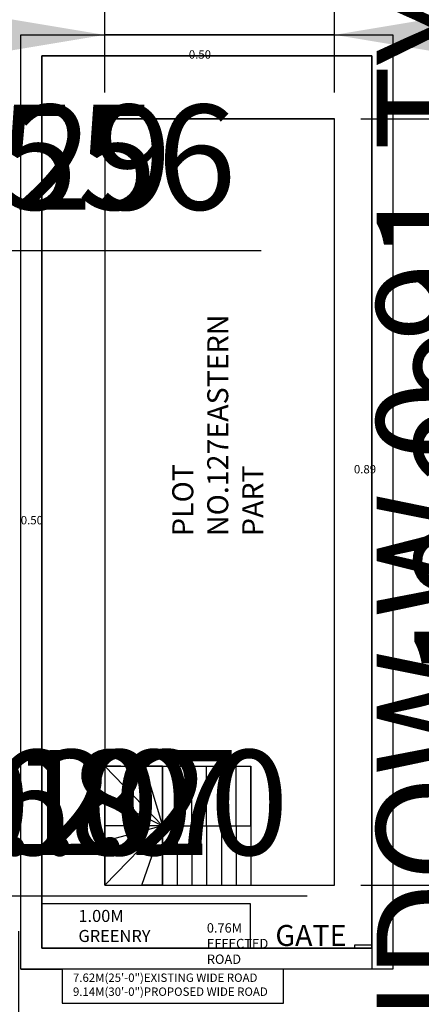
# Model space of a CAD drawing. Units: metres. Extents: x 782 to 1487, y 1262 to 7446.
# Tile 22 of 25: x 816.33 to 825.91, y 1313.5 to 1336.99. Entities that reach past the tile are written whole.
import ezdxf

# ---------------------------------------------------------------- set-up
doc = ezdxf.new("R2010")
doc.units = ezdxf.units.M
for name, color, linetype, lineweight in [('A-ANNO-DIMS', 2, 'Continuous', 18), ('A-ANNO-TEXT', 3, 'Continuous', 18), ('C-PROP', 6, 'Continuous', 25)]:
    doc.layers.add(name, color=color, linetype=linetype, lineweight=lineweight)
doc.styles.get("Standard").update_dxf_attribs({"font": 'arial.ttf'})
doc.dimstyles.new('ISO-25', dxfattribs={"dimtxt": 2.5, "dimasz": 2.5, "dimexe": 1.25, "dimexo": 0.625, "dimtad": 1, "dimtxsty": 'Standard', "dimcen": 2.5, "dimadec": 0, "dimazin": 0, "dimtfac": 1, "dimtmove": 0, "dimatfit": 3, "dimfxl": 1, "dimarcsym": 0})

# ---------------------------------------------------------------- blocks, each defined once
blk = doc.blocks.new('*D11')
at = {"layer": 'A-ANNO-DIMS', "color": 0, "lineweight": -2, "transparency": 16777216}
for p, q in [((824.462, 1334.623), (830.687, 1334.623)), ((829.437, 1332.123), (829.437, 1318.837)), ((824.462, 1316.337), (830.687, 1316.337))]:
    blk.add_line(p, q, dxfattribs=at)
at = {"layer": 'A-ANNO-DIMS', "color": 0, "transparency": 16777216}
for points in [[(829.02, 1332.123), (829.854, 1332.123), (829.437, 1334.623)], [(829.02, 1318.837), (829.854, 1318.837), (829.437, 1316.337)]]:
    blk.add_solid(points, dxfattribs=at)
at = {"layer": 'Defpoints', "color": 0, "transparency": 16777216}
for p in [(823.837, 1334.623), (823.837, 1316.337), (829.437, 1316.337)]:
    blk.add_point(p, dxfattribs=at)
at = {"layer": 'A-ANNO-DIMS', "color": 0, "transparency": 16777216, "insert": (827.31, 1325.48), "char_height": 2.5, "attachment_point": 5, "rotation": 90}
blk.add_mtext('18,29', dxfattribs=at)
blk = doc.blocks.new('*D12')
at = {"layer": 'A-ANNO-DIMS', "color": 0, "lineweight": -2, "transparency": 16777216}
for p, q in [((818.357, 1335.252), (818.357, 1337.877)), ((823.837, 1335.252), (823.837, 1337.877)), ((815.857, 1336.627), (805.608, 1336.627)), ((823.837, 1336.627), (818.357, 1336.627)), ((826.337, 1336.627), (828.837, 1336.627))]:
    blk.add_line(p, q, dxfattribs=at)
at = {"layer": 'A-ANNO-DIMS', "color": 0, "transparency": 16777216}
for points in [[(815.857, 1337.044), (815.857, 1336.21), (818.357, 1336.627)], [(826.337, 1337.044), (826.337, 1336.21), (823.837, 1336.627)]]:
    blk.add_solid(points, dxfattribs=at)
at = {"layer": 'Defpoints', "color": 0, "transparency": 16777216}
for p in [(818.357, 1336.627), (818.357, 1334.627), (823.837, 1334.627)]:
    blk.add_point(p, dxfattribs=at)
at = {"layer": 'A-ANNO-DIMS', "color": 0, "transparency": 16777216, "insert": (809.482, 1338.754), "char_height": 2.5, "width": 6.51678, "attachment_point": 5}
blk.add_mtext('5,48', dxfattribs=at)
blk = doc.blocks.new('*D20')
at = {"layer": 'A-ANNO-DIMS', "color": 0, "lineweight": -2, "transparency": 16777216}
for p, q in [((831.056, 1302.088), (831.056, 1337.678)), ((831.056, 1298.698), (831.056, 1299.588)), ((831.548, 1299.588), (832.306, 1299.588)), ((831.548, 1298.698), (832.306, 1298.698)), ((831.056, 1296.198), (831.056, 1293.698))]:
    blk.add_line(p, q, dxfattribs=at)
at = {"layer": 'A-ANNO-DIMS', "color": 0, "transparency": 16777216}
for points in [[(830.64, 1302.088), (831.473, 1302.088), (831.056, 1299.588)], [(830.64, 1296.198), (831.473, 1296.198), (831.056, 1298.698)]]:
    blk.add_solid(points, dxfattribs=at)
at = {"layer": 'Defpoints', "color": 0, "transparency": 16777216}
for p in [(830.923, 1299.588), (831.056, 1299.588), (830.923, 1298.698)]:
    blk.add_point(p, dxfattribs=at)
at = {"layer": 'A-ANNO-DIMS', "color": 0, "transparency": 16777216, "insert": (829.138, 1321.133), "char_height": 2.5, "attachment_point": 5, "rotation": 90}
blk.add_mtext('DOOR D1 0.89 TYP.', dxfattribs=at)
blk = doc.blocks.new('*D23')
at = {"layer": 'A-ANNO-DIMS', "color": 0, "lineweight": -2, "transparency": 16777216}
for p, q in [((816.313, 1296.414), (816.313, 1315.246)), ((816.313, 1293.067), (816.313, 1293.914)), ((816.804, 1293.914), (817.563, 1293.914)), ((816.804, 1293.067), (817.563, 1293.067)), ((816.313, 1290.567), (816.313, 1288.067))]:
    blk.add_line(p, q, dxfattribs=at)
at = {"layer": 'A-ANNO-DIMS', "color": 0, "transparency": 16777216}
for points in [[(815.896, 1296.414), (816.729, 1296.414), (816.313, 1293.914)], [(815.896, 1290.567), (816.729, 1290.567), (816.313, 1293.067)]]:
    blk.add_solid(points, dxfattribs=at)
at = {"layer": 'Defpoints', "color": 0, "transparency": 16777216}
for p in [(816.179, 1293.914), (816.313, 1293.914), (816.179, 1293.067)]:
    blk.add_point(p, dxfattribs=at)
at = {"layer": 'A-ANNO-DIMS', "color": 0, "transparency": 16777216, "insert": (814.411, 1307.08), "char_height": 2.5, "attachment_point": 5, "rotation": 90}
blk.add_mtext('0.85 TYP.', dxfattribs=at)
blk = doc.blocks.new('*D25')
at = {"layer": 'A-ANNO-DIMS', "color": 0, "lineweight": -2, "transparency": 16777216}
for p, q in [((814.687, 1297.897), (814.687, 1316.729)), ((814.687, 1294.551), (814.687, 1295.397)), ((815.184, 1295.397), (815.937, 1295.397)), ((815.184, 1294.551), (815.937, 1294.551)), ((814.687, 1292.051), (814.687, 1289.551))]:
    blk.add_line(p, q, dxfattribs=at)
at = {"layer": 'A-ANNO-DIMS', "color": 0, "transparency": 16777216}
for points in [[(814.27, 1297.897), (815.103, 1297.897), (814.687, 1295.397)], [(814.27, 1292.051), (815.103, 1292.051), (814.687, 1294.551)]]:
    blk.add_solid(points, dxfattribs=at)
at = {"layer": 'Defpoints', "color": 0, "transparency": 16777216}
for p in [(814.559, 1295.397), (814.687, 1295.397), (814.559, 1294.551)]:
    blk.add_point(p, dxfattribs=at)
at = {"layer": 'A-ANNO-DIMS', "color": 0, "transparency": 16777216, "insert": (812.785, 1308.563), "char_height": 2.5, "attachment_point": 5, "rotation": 90}
blk.add_mtext('0.85 TYP.', dxfattribs=at)
blk = doc.blocks.new('*D26')
at = {"layer": 'A-ANNO-DIMS', "color": 0, "lineweight": -2, "transparency": 16777216}
for p, q in [((828.33, 1303.223), (828.33, 1342.718)), ((828.33, 1299.809), (828.33, 1300.723)), ((828.818, 1300.723), (829.58, 1300.723)), ((828.818, 1299.809), (829.58, 1299.809)), ((828.33, 1297.309), (828.33, 1294.809))]:
    blk.add_line(p, q, dxfattribs=at)
at = {"layer": 'A-ANNO-DIMS', "color": 0, "transparency": 16777216}
for points in [[(827.913, 1303.223), (828.747, 1303.223), (828.33, 1300.723)], [(827.913, 1297.309), (828.747, 1297.309), (828.33, 1299.809)]]:
    blk.add_solid(points, dxfattribs=at)
at = {"layer": 'Defpoints', "color": 0, "transparency": 16777216}
for p in [(828.193, 1300.723), (828.33, 1300.723), (828.193, 1299.809)]:
    blk.add_point(p, dxfattribs=at)
at = {"layer": 'A-ANNO-DIMS', "color": 0, "transparency": 16777216, "insert": (826.412, 1324.22), "char_height": 2.5, "attachment_point": 5, "rotation": 90}
blk.add_mtext('WINDOW W 0.91 TYP.', dxfattribs=at)
blk = doc.blocks.new('*D28')
at = {"layer": 'A-ANNO-DIMS', "color": 0, "lineweight": -2, "transparency": 16777216}
for p, q in [((832.55, 1308.281), (832.55, 1349.718)), ((832.55, 1304.867), (832.55, 1305.781)), ((833.038, 1305.781), (833.8, 1305.781)), ((833.038, 1304.867), (833.8, 1304.867)), ((832.55, 1302.367), (832.55, 1299.867))]:
    blk.add_line(p, q, dxfattribs=at)
at = {"layer": 'A-ANNO-DIMS', "color": 0, "transparency": 16777216}
for points in [[(832.134, 1308.281), (832.967, 1308.281), (832.55, 1305.781)], [(832.134, 1302.367), (832.967, 1302.367), (832.55, 1304.867)]]:
    blk.add_solid(points, dxfattribs=at)
at = {"layer": 'Defpoints', "color": 0, "transparency": 16777216}
for p in [(832.413, 1305.781), (832.55, 1305.781), (832.413, 1304.867)]:
    blk.add_point(p, dxfattribs=at)
at = {"layer": 'A-ANNO-DIMS', "color": 0, "transparency": 16777216, "insert": (830.632, 1330.25), "char_height": 2.5, "attachment_point": 5, "rotation": 90}
blk.add_mtext('WINDOW W1 0.91 TYP.', dxfattribs=at)
blk = doc.blocks.new('*D137')
at = {"layer": 'A-ANNO-DIMS', "color": 0, "lineweight": -2, "transparency": 16777216}
for p, q in [((803.332, 1330.988), (803.332, 1332.733)), ((809.888, 1330.988), (809.888, 1332.733)), ((805.832, 1331.483), (807.388, 1331.483)), ((809.888, 1331.483), (822.086, 1331.483))]:
    blk.add_line(p, q, dxfattribs=at)
at = {"layer": 'A-ANNO-DIMS', "color": 0, "transparency": 16777216}
for points in [[(805.832, 1331.899), (805.832, 1331.066), (803.332, 1331.483)], [(807.388, 1331.899), (807.388, 1331.066), (809.888, 1331.483)]]:
    blk.add_solid(points, dxfattribs=at)
at = {"layer": 'Defpoints', "color": 0, "transparency": 16777216}
for p in [(809.888, 1331.483), (803.332, 1330.363), (809.888, 1330.363)]:
    blk.add_point(p, dxfattribs=at)
at = {"layer": 'A-ANNO-DIMS', "color": 0, "transparency": 16777216, "insert": (817.237, 1333.384), "char_height": 2.5, "attachment_point": 5}
blk.add_mtext('6.556', dxfattribs=at)
blk = doc.blocks.new('*D139')
at = {"layer": 'A-ANNO-DIMS', "color": 0, "lineweight": -2, "transparency": 16777216}
for p, q in [((807.481, 1330.074), (807.481, 1332.733)), ((807.769, 1330.074), (807.769, 1332.733)), ((804.981, 1331.483), (802.481, 1331.483)), ((807.481, 1331.483), (807.769, 1331.483)), ((810.269, 1331.483), (820.518, 1331.483))]:
    blk.add_line(p, q, dxfattribs=at)
at = {"layer": 'A-ANNO-DIMS', "color": 0, "transparency": 16777216}
for points in [[(804.981, 1331.899), (804.981, 1331.066), (807.481, 1331.483)], [(810.269, 1331.899), (810.269, 1331.066), (807.769, 1331.483)]]:
    blk.add_solid(points, dxfattribs=at)
at = {"layer": 'Defpoints', "color": 0, "transparency": 16777216}
for p in [(807.769, 1331.483), (807.481, 1329.449), (807.769, 1329.449)]:
    blk.add_point(p, dxfattribs=at)
at = {"layer": 'A-ANNO-DIMS', "color": 0, "transparency": 16777216, "insert": (816.644, 1333.384), "char_height": 2.5, "attachment_point": 5}
blk.add_mtext('0.29', dxfattribs=at)
blk = doc.blocks.new('*D140')
at = {"layer": 'A-ANNO-DIMS', "color": 0, "lineweight": -2, "transparency": 16777216}
for p, q in [((803.316, 1317.905), (803.316, 1314.838)), ((804.52, 1317.905), (804.52, 1314.838)), ((800.816, 1316.088), (798.316, 1316.088)), ((803.316, 1316.088), (804.52, 1316.088)), ((807.02, 1316.088), (817.02, 1316.088))]:
    blk.add_line(p, q, dxfattribs=at)
at = {"layer": 'A-ANNO-DIMS', "color": 0, "transparency": 16777216}
for points in [[(800.816, 1316.505), (800.816, 1315.671), (803.316, 1316.088)], [(807.02, 1316.505), (807.02, 1315.671), (804.52, 1316.088)]]:
    blk.add_solid(points, dxfattribs=at)
at = {"layer": 'Defpoints', "color": 0, "transparency": 16777216}
for p in [(803.316, 1318.53), (804.52, 1318.53), (804.52, 1316.088)]:
    blk.add_point(p, dxfattribs=at)
at = {"layer": 'A-ANNO-DIMS', "color": 0, "transparency": 16777216, "insert": (813.27, 1317.989), "char_height": 2.5, "attachment_point": 5}
blk.add_mtext('1.20', dxfattribs=at)
blk = doc.blocks.new('*D141')
at = {"layer": 'A-ANNO-DIMS', "color": 0, "lineweight": -2, "transparency": 16777216}
for p, q in [((804.52, 1317.905), (804.52, 1314.838)), ((807.205, 1317.905), (807.205, 1314.838)), ((802.02, 1316.088), (799.52, 1316.088)), ((804.52, 1316.088), (807.205, 1316.088)), ((809.705, 1316.088), (819.997, 1316.088))]:
    blk.add_line(p, q, dxfattribs=at)
at = {"layer": 'A-ANNO-DIMS', "color": 0, "transparency": 16777216}
for points in [[(802.02, 1316.505), (802.02, 1315.671), (804.52, 1316.088)], [(809.705, 1316.505), (809.705, 1315.671), (807.205, 1316.088)]]:
    blk.add_solid(points, dxfattribs=at)
at = {"layer": 'Defpoints', "color": 0, "transparency": 16777216}
for p in [(804.52, 1318.53), (807.205, 1318.53), (807.205, 1316.088)]:
    blk.add_point(p, dxfattribs=at)
at = {"layer": 'A-ANNO-DIMS', "color": 0, "transparency": 16777216, "insert": (816.101, 1317.989), "char_height": 2.5, "attachment_point": 5}
blk.add_mtext('2.68', dxfattribs=at)
blk = doc.blocks.new('*D142')
at = {"layer": 'A-ANNO-DIMS', "color": 0, "lineweight": -2, "transparency": 16777216}
for p, q in [((807.205, 1317.905), (807.205, 1314.838)), ((808.409, 1317.905), (808.409, 1314.838)), ((804.705, 1316.088), (802.205, 1316.088)), ((807.205, 1316.088), (808.409, 1316.088)), ((810.909, 1316.088), (820.909, 1316.088))]:
    blk.add_line(p, q, dxfattribs=at)
at = {"layer": 'A-ANNO-DIMS', "color": 0, "transparency": 16777216}
for points in [[(804.705, 1316.505), (804.705, 1315.671), (807.205, 1316.088)], [(810.909, 1316.505), (810.909, 1315.671), (808.409, 1316.088)]]:
    blk.add_solid(points, dxfattribs=at)
at = {"layer": 'Defpoints', "color": 0, "transparency": 16777216}
for p in [(807.205, 1318.53), (808.409, 1318.53), (808.409, 1316.088)]:
    blk.add_point(p, dxfattribs=at)
at = {"layer": 'A-ANNO-DIMS', "color": 0, "transparency": 16777216, "insert": (817.159, 1317.989), "char_height": 2.5, "attachment_point": 5}
blk.add_mtext('1.20', dxfattribs=at)
blk = doc.blocks.new('*D143')
at = {"layer": 'A-ANNO-DIMS', "color": 0, "lineweight": -2, "transparency": 16777216}
for p, q in [((808.409, 1317.905), (808.409, 1314.838)), ((809.479, 1317.905), (809.479, 1314.838)), ((805.909, 1316.088), (803.409, 1316.088)), ((808.409, 1316.088), (809.479, 1316.088)), ((811.979, 1316.088), (821.987, 1316.088))]:
    blk.add_line(p, q, dxfattribs=at)
at = {"layer": 'A-ANNO-DIMS', "color": 0, "transparency": 16777216}
for points in [[(805.909, 1316.505), (805.909, 1315.671), (808.409, 1316.088)], [(811.979, 1316.505), (811.979, 1315.671), (809.479, 1316.088)]]:
    blk.add_solid(points, dxfattribs=at)
at = {"layer": 'Defpoints', "color": 0, "transparency": 16777216}
for p in [(808.409, 1318.53), (809.479, 1318.53), (809.479, 1316.088)]:
    blk.add_point(p, dxfattribs=at)
at = {"layer": 'A-ANNO-DIMS', "color": 0, "transparency": 16777216, "insert": (818.233, 1317.989), "char_height": 2.5, "attachment_point": 5}
blk.add_mtext('1.07', dxfattribs=at)
blk = doc.blocks.new('*D144')
at = {"layer": 'A-ANNO-DIMS', "color": 0, "lineweight": -2, "transparency": 16777216}
for p, q in [((809.479, 1317.905), (809.479, 1314.838)), ((810.683, 1317.905), (810.683, 1314.838)), ((806.979, 1316.088), (804.479, 1316.088)), ((809.479, 1316.088), (810.683, 1316.088)), ((813.183, 1316.088), (823.183, 1316.088))]:
    blk.add_line(p, q, dxfattribs=at)
at = {"layer": 'A-ANNO-DIMS', "color": 0, "transparency": 16777216}
for points in [[(806.979, 1316.505), (806.979, 1315.671), (809.479, 1316.088)], [(813.183, 1316.505), (813.183, 1315.671), (810.683, 1316.088)]]:
    blk.add_solid(points, dxfattribs=at)
at = {"layer": 'Defpoints', "color": 0, "transparency": 16777216}
for p in [(809.479, 1318.53), (810.683, 1318.53), (810.683, 1316.088)]:
    blk.add_point(p, dxfattribs=at)
at = {"layer": 'A-ANNO-DIMS', "color": 0, "transparency": 16777216, "insert": (819.433, 1317.989), "char_height": 2.5, "attachment_point": 5}
blk.add_mtext('1.20', dxfattribs=at)

msp = doc.modelspace()

# ---------------------------------------------------------------- linework, layer by layer
at = {"layer": 'C-PROP'}
for p, q in [((824.727, 1336.127), (816.857, 1336.127)), ((816.857, 1336.127), (816.857, 1316.337)), ((824.727, 1316.337), (824.727, 1336.127)), ((823.837, 1334.627), (818.357, 1334.627)), ((818.357, 1334.627), (818.357, 1316.337)), ((818.357, 1334.627), (823.837, 1334.627)), ((818.357, 1334.627), (818.6097, 1334.627)), ((818.6097, 1334.627), (818.357, 1334.627)), ((823.4498, 1334.6231), (823.8366, 1334.6231)), ((823.837, 1316.337), (823.837, 1334.627)), ((823.837, 1316.337), (823.837, 1334.627)), ((818.7439, 1319.1768), (818.357, 1319.1768)), ((818.357, 1319.1768), (821.1122, 1319.1768)), ((819.7346, 1317.7569), (818.357, 1319.1768)), ((819.7346, 1319.1768), (819.309, 1319.1768)), ((819.309, 1319.1768), (819.7346, 1317.7569)), ((819.7346, 1319.1768), (819.7346, 1316.337)), ((819.7346, 1317.7569), (819.7346, 1319.1768)), ((819.7346, 1316.337), (819.7346, 1319.1768)), ((819.7346, 1317.7569), (819.7346, 1319.1768)), ((820.0859, 1317.7569), (820.0859, 1319.1768)), ((820.4371, 1317.7569), (820.4371, 1319.1768)), ((820.7883, 1317.7569), (820.7883, 1319.1768)), ((821.1122, 1319.1768), (821.842, 1319.1768)), ((821.1396, 1317.7569), (821.1396, 1319.1768)), ((821.4908, 1317.7569), (821.4908, 1319.1768)), ((821.842, 1319.1768), (821.842, 1316.337)), ((821.842, 1317.7569), (821.842, 1319.1768)), ((818.357, 1316.337), (818.357, 1318.4398)), ((818.357, 1318.4398), (819.7346, 1317.7569)), ((819.7346, 1317.7569), (818.357, 1317.7569)), ((819.7346, 1317.7569), (818.357, 1317.7569)), ((819.7346, 1317.7569), (818.357, 1316.337)), ((819.7346, 1317.7569), (818.357, 1316.337)), ((819.7346, 1317.7569), (818.357, 1317.3884)), ((819.2441, 1316.337), (819.7346, 1317.7569)), ((819.7346, 1317.7569), (821.842, 1317.7569)), ((819.7346, 1317.7569), (821.842, 1317.7569)), ((819.7346, 1317.7569), (819.7346, 1316.337)), ((819.7346, 1317.7569), (819.7346, 1316.337)), ((820.0859, 1317.7569), (820.0859, 1316.337)), ((820.4371, 1317.7569), (820.4371, 1316.337)), ((820.7883, 1317.7569), (820.7883, 1316.337)), ((821.1396, 1317.7569), (821.1396, 1316.337)), ((821.4908, 1317.7569), (821.4908, 1316.337)), ((816.857, 1316.337), (816.857, 1314.837)), ((816.857, 1316.337), (816.857, 1315.9019)), ((818.357, 1316.337), (823.837, 1316.337)), ((818.357, 1316.337), (822.947, 1316.337)), ((818.357, 1316.337), (823.837, 1316.337)), ((818.357, 1316.337), (821.1122, 1316.337)), ((819.7346, 1316.337), (819.2441, 1316.337)), ((821.1122, 1316.337), (821.842, 1316.337)), ((824.727, 1314.837), (824.727, 1316.337)), ((816.857, 1315.9019), (821.8225, 1315.9019)), ((821.8225, 1315.9019), (821.8225, 1314.837)), ((816.857, 1314.837), (824.727, 1314.837)), ((824.727, 1314.9097), (824.315, 1314.9097)), ((824.315, 1314.9097), (824.315, 1314.837)), ((824.727, 1314.837), (824.727, 1314.9097)), ((824.727, 1314.837), (824.727, 1314.337)), ((816.357, 1314.337), (817.3441, 1314.337)), ((817.3441, 1314.337), (817.3441, 1313.5272)), ((822.6209, 1313.5272), (822.6209, 1314.337)), ((817.3441, 1313.5272), (822.6209, 1313.5272))]:
    msp.add_line(p, q, dxfattribs=at)
for points in [[(816.357, 1336.627), (825.227, 1336.627), (825.227, 1314.337), (816.357, 1314.337)], [(816.857, 1336.127), (824.727, 1336.127), (824.727, 1314.837), (816.857, 1314.837)]]:
    msp.add_lwpolyline(points, close=True, dxfattribs=at)

# ---------------------------------------------------------------- texts
at = {"layer": 'A-ANNO-TEXT', "attachment_point": 1}
for s, width, gutter_width, insert, char_height in [('\\P0.50 ', 2, 12.5, (820.363, 1336.5927), 0.2), ('\\P0.89', 2, 12.5, (824.298, 1326.6977), 0.2), ('\\P0.50 ', 2, 12.5, (816.357, 1325.482), 0.2), ('1.00M GREENRY ', 1.868468, 7.1702, (817.7312, 1315.7494), 0.28681), ('0.76M EFFECTED ROAD', 0.958525, 5.5983, (820.792, 1315.4326), 0.223933), ('\\PGATE', 1.863436, 12.5, (822.4264, 1316.2235), 0.5), ('\\P7.62M(25\'-0")EXISTING WIDE ROAD\\P9.14M(30\'-0")PROPOSED WIDE ROAD', 8.739904, 12.5, (817.6007, 1314.5661), 0.2)]:
    msp.add_mtext_dynamic_manual_height_columns(s, width=width, gutter_width=gutter_width, heights=[0], dxfattribs=dict(at, insert=insert, char_height=char_height))
at = {"layer": 'A-ANNO-TEXT', "insert": (819.9694, 1324.6695), "char_height": 0.5, "attachment_point": 1, "rotation": 90}
msp.add_mtext_dynamic_manual_height_columns('PLOT NO.127EASTERN PART', width=4.107799, gutter_width=12.5, heights=[0], dxfattribs=at)

# ---------------------------------------------------------------- dimensions: what is measured, and where the dimension line sits
at = {"layer": 'A-ANNO-DIMS'}
for base, p1, p2, text, picture, middle in [((832.5503, 1305.7809), (832.4132, 1304.8669), (832.4132, 1305.7809), 'WINDOW W1 <> TYP.', '*D28', (830.6318, 1330.2497)), ((828.3302, 1300.7228), (828.1931, 1299.8088), (828.1931, 1300.7228), 'WINDOW W <> TYP.', '*D26', (826.4117, 1324.2204)), ((831.0564, 1299.5877), (830.923, 1298.6982), (830.923, 1299.5877), 'DOOR D1 <> TYP.', '*D20', (829.138, 1321.1327)), ((814.6868, 1295.3974), (814.5592, 1294.5507), (814.5592, 1295.3974), '<> TYP.', '*D25', (812.7854, 1308.5633)), ((816.3126, 1293.9141), (816.1792, 1293.0674), (816.1792, 1293.9141), '<> TYP.', '*D23', (814.4112, 1307.08))]:
    dim = msp.add_linear_dim(base=base, p1=p1, p2=p2, angle=90, text=text, dimstyle='ISO-25', override={"dimdec": 2, "dimlfac": 1, "dimrnd": 0, "dimzin": 0, "dimdsep": 46, "dimlunit": 2}, dxfattribs=at)
    dim.commit()
    dim.dimension.update_dxf_attribs({"geometry": picture, "text_midpoint": middle})
for base, p1, p2, override, picture, middle in [((818.357, 1336.627), (823.837, 1334.627), (818.357, 1334.627), {"dimclrd": 0, "dimclre": 0, "dimclrt": 0}, '*D12', (809.4825, 1338.7544)), ((807.7695, 1331.4828), (807.4812, 1329.4495), (807.7695, 1329.4495), {"dimdec": 2, "dimlfac": 1, "dimrnd": 0, "dimzin": 0, "dimdsep": 46, "dimlunit": 2}, '*D139', (816.6439, 1333.3843)), ((809.8881, 1331.4828), (803.3321, 1330.3635), (809.8881, 1330.3635), {"dimdec": 3, "dimlfac": 1, "dimrnd": 0, "dimzin": 0, "dimdsep": 46, "dimlunit": 2}, '*D137', (817.2371, 1333.3843)), ((804.5202, 1316.088), (803.3164, 1318.53), (804.5202, 1318.53), {"dimdec": 2, "dimlfac": 1, "dimrnd": 0, "dimzin": 0, "dimdsep": 46, "dimlunit": 2}, '*D140', (813.2702, 1317.9895)), ((807.205, 1316.088), (804.5202, 1318.53), (807.205, 1318.53), {"dimdec": 2, "dimlfac": 1, "dimrnd": 0, "dimzin": 0, "dimdsep": 46, "dimlunit": 2}, '*D141', (816.1008, 1317.9895)), ((808.4088, 1316.088), (807.205, 1318.53), (808.4088, 1318.53), {"dimdec": 2, "dimlfac": 1, "dimrnd": 0, "dimzin": 0, "dimdsep": 46, "dimlunit": 2}, '*D142', (817.1588, 1317.9895)), ((809.4788, 1316.088), (808.4088, 1318.53), (809.4788, 1318.53), {"dimdec": 2, "dimlfac": 1, "dimrnd": 0, "dimzin": 0, "dimdsep": 46, "dimlunit": 2}, '*D143', (818.2331, 1317.9895)), ((810.6826, 1316.088), (809.4788, 1318.53), (810.6826, 1318.53), {"dimdec": 2, "dimlfac": 1, "dimrnd": 0, "dimzin": 0, "dimdsep": 46, "dimlunit": 2}, '*D144', (819.4326, 1317.9895))]:
    dim = msp.add_linear_dim(base=base, p1=p1, p2=p2, dimstyle='ISO-25', override=override, dxfattribs=at)
    dim.commit()
    dim.dimension.update_dxf_attribs({"geometry": picture, "text_midpoint": middle})
dim = msp.add_linear_dim(base=(829.437, 1316.337), p1=(823.8366, 1334.6231), p2=(823.8366, 1316.337), angle=90, dimstyle='ISO-25', override={"dimclrd": 0, "dimclre": 0, "dimclrt": 0}, dxfattribs=at)
dim.commit()
dim.dimension.update_dxf_attribs({"geometry": '*D11', "text_midpoint": (827.3096, 1325.48)})

doc.saveas('drawing.dxf')
